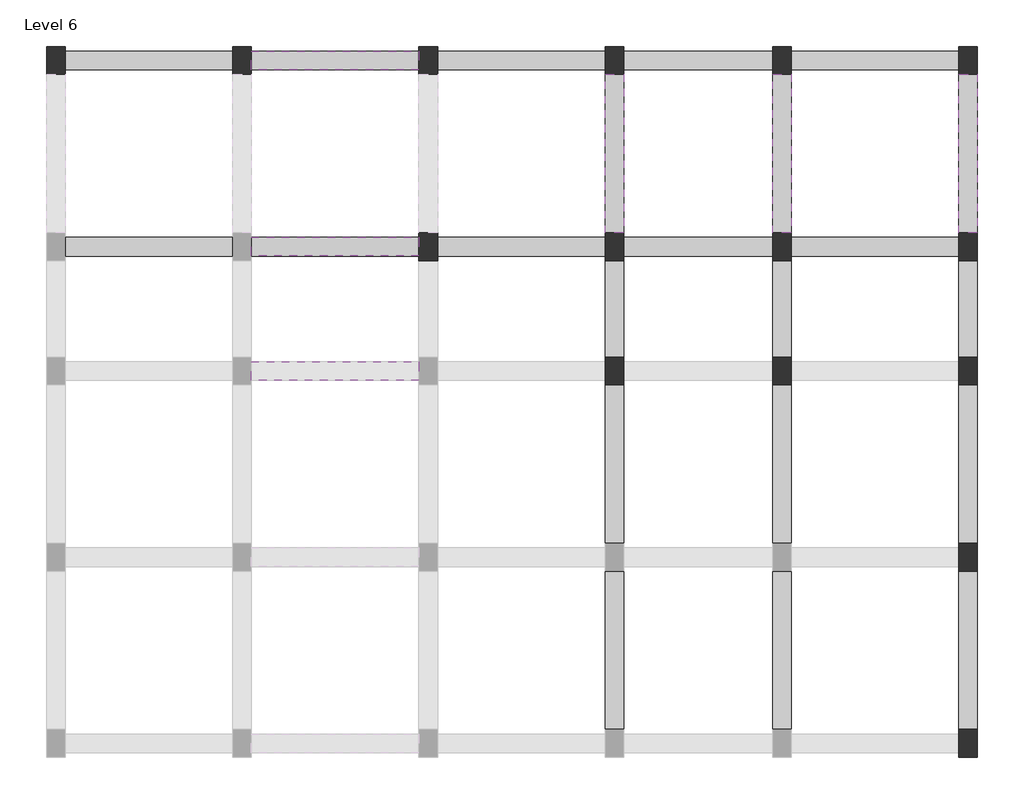
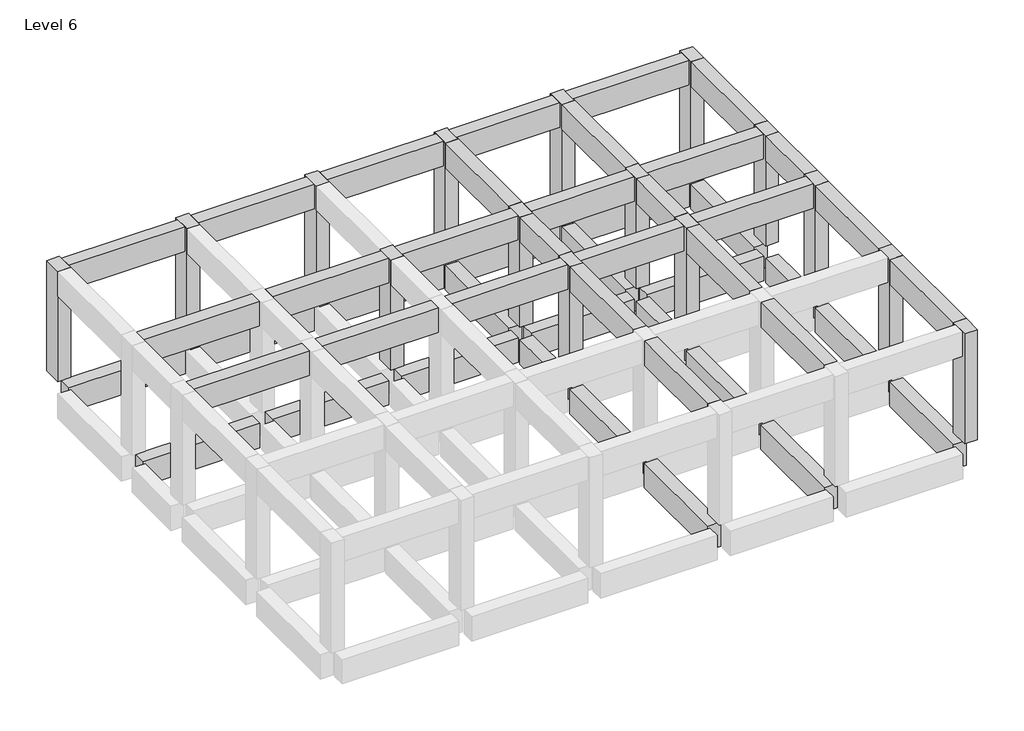
# One storey, part 2 of 2: 15 columns, 11 beams.
"""IFC4 building model written with IfcOpenShell, lengths in millimetres."""

from ifc_helpers import new_model, si_unit, frame, origin, place, context, project, spatial, polyline, outline, extrude, faceted_brep, element, save

model = new_model("IFC4")

# Units and contexts
model_context = context("Model", 3, world=origin())
ifc_project = project(units=[si_unit("LENGTHUNIT", "METRE", prefix="MILLI")], contexts=[model_context])

# Site, building, storey
site = spatial("IfcSite", under=ifc_project)
building = spatial("IfcBuilding", under=site)
storey = spatial("IfcBuildingStorey", under=building, Name="Level 6", Elevation=15240.0)

# Beams
placement = place(None, origin())
element("IfcBeam", 1, ObjectType="Concrete-Rectangular Beam : 12 x 24", at=placement, inside=storey, context=model_context, shape_type="SweptSolid", body=[
    extrude(outline(polyline([(2607.7603583, 15727.9119241), (2607.7603583, 15423.1119241), (-135.4396417, 15423.1119241), (-135.4396417, 15727.9119241), (2607.7603583, 15727.9119241)])), frame((0.0, 0.0, 14325.6), z_axis=(0.0, 0.0, 1.0), x_axis=(1.0, 0.0, 0.0)), (0.0, 0.0, 1.0), 609.6),
    extrude(outline(polyline([(-12022.6396417, 15423.1119241), (-12022.6396417, 15727.9119241), (-9279.4396417, 15727.9119241), (-9279.4396417, 15423.1119241), (-12022.6396417, 15423.1119241)])), frame((0.0, 0.0, 14325.6), z_axis=(0.0, 0.0, 1.0), x_axis=(1.0, 0.0, 0.0)), (0.0, 0.0, 1.0), 609.6),
    extrude(outline(polyline([(-8974.6396417, 15423.1119241), (-8974.6396417, 15727.9119241), (-6231.4396417, 15727.9119241), (-6231.4396417, 15423.1119241), (-8974.6396417, 15423.1119241)])), frame((0.0, 0.0, 14325.6), z_axis=(0.0, 0.0, 1.0), x_axis=(1.0, 0.0, 0.0)), (0.0, 0.0, 1.0), 609.6),
    extrude(outline(polyline([(-5926.6396417, 15423.1119241), (-5926.6396417, 15727.9119241), (-3183.4396417, 15727.9119241), (-3183.4396417, 15423.1119241), (-5926.6396417, 15423.1119241)])), frame((0.0, 0.0, 14325.6), z_axis=(0.0, 0.0, 1.0), x_axis=(1.0, 0.0, 0.0)), (0.0, 0.0, 1.0), 609.6),
    extrude(outline(polyline([(-2878.6396417, 15423.1119241), (-2878.6396417, 15727.9119241), (-440.2396417, 15727.9119241), (-440.2396417, 15423.1119241), (-2878.6396417, 15423.1119241)])), frame((0.0, 0.0, 14325.6), z_axis=(0.0, 0.0, 1.0), x_axis=(1.0, 0.0, 0.0)), (0.0, 0.0, 1.0), 609.6),
])
element("IfcBeam", 2, ObjectType="Concrete-Rectangular Beam : 12 x 24", at=placement, inside=storey, context=model_context, shape_type="SweptSolid", body=[
    extrude(outline(polyline([(2607.7603583, 18775.9119241), (2607.7603583, 18471.1119241), (-135.4396417, 18471.1119241), (-135.4396417, 18775.9119241), (2607.7603583, 18775.9119241)])), frame((0.0, 0.0, 14325.6), z_axis=(0.0, 0.0, 1.0), x_axis=(1.0, 0.0, 0.0)), (0.0, 0.0, 1.0), 609.6),
    extrude(outline(polyline([(-12022.6396417, 18471.1119241), (-12022.6396417, 18775.9119241), (-9279.4396417, 18775.9119241), (-9279.4396417, 18471.1119241), (-12022.6396417, 18471.1119241)])), frame((0.0, 0.0, 14325.6), z_axis=(0.0, 0.0, 1.0), x_axis=(1.0, 0.0, 0.0)), (0.0, 0.0, 1.0), 609.6),
    extrude(outline(polyline([(-8974.6396417, 18471.1119241), (-8974.6396417, 18775.9119241), (-6231.4396417, 18775.9119241), (-6231.4396417, 18471.1119241), (-8974.6396417, 18471.1119241)])), frame((0.0, 0.0, 14325.6), z_axis=(0.0, 0.0, 1.0), x_axis=(1.0, 0.0, 0.0)), (0.0, 0.0, 1.0), 609.6),
    extrude(outline(polyline([(-5926.6396417, 18471.1119241), (-5926.6396417, 18775.9119241), (-3183.4396417, 18775.9119241), (-3183.4396417, 18471.1119241), (-5926.6396417, 18471.1119241)])), frame((0.0, 0.0, 14325.6), z_axis=(0.0, 0.0, 1.0), x_axis=(1.0, 0.0, 0.0)), (0.0, 0.0, 1.0), 609.6),
    extrude(outline(polyline([(-2878.6396417, 18471.1119241), (-2878.6396417, 18775.9119241), (-440.2396417, 18775.9119241), (-440.2396417, 18471.1119241), (-2878.6396417, 18471.1119241)])), frame((0.0, 0.0, 14325.6), z_axis=(0.0, 0.0, 1.0), x_axis=(1.0, 0.0, 0.0)), (0.0, 0.0, 1.0), 609.6),
])
element("IfcBeam", 3, ObjectType="Concrete-Rectangular Beam : 12 x 24", at=placement, inside=storey, context=model_context, shape_type="SweptSolid", body=[
    extrude(outline(polyline([(-2878.6396417, 7672.8647757), (-3183.4396417, 7672.8647757), (-3183.4396417, 10263.6647757), (-2878.6396417, 10263.6647757), (-2878.6396417, 7672.8647757)])), frame((0.0, 0.0, 14325.6), z_axis=(0.0, 0.0, 1.0), x_axis=(1.0, 0.0, 0.0)), (0.0, 0.0, 1.0), 609.6),
    extrude(outline(polyline([(-3183.4396417, 18394.9119241), (-2878.6396417, 18394.9119241), (-2878.6396417, 15804.1119241), (-3183.4396417, 15804.1119241), (-3183.4396417, 18394.9119241)])), frame((0.0, 0.0, 14325.6), z_axis=(0.0, 0.0, 1.0), x_axis=(1.0, 0.0, 0.0)), (0.0, 0.0, 1.0), 609.6),
    extrude(outline(polyline([(-2878.6396417, 10720.8647757), (-3183.4396417, 10720.8647757), (-3183.4396417, 13311.6647757), (-2878.6396417, 13311.6647757), (-2878.6396417, 10720.8647757)])), frame((0.0, 0.0, 14325.6), z_axis=(0.0, 0.0, 1.0), x_axis=(1.0, 0.0, 0.0)), (0.0, 0.0, 1.0), 609.6),
    extrude(outline(polyline([(-2878.6396417, 13768.8647757), (-3183.4396417, 13768.8647757), (-3183.4396417, 15346.9119241), (-2878.6396417, 15346.9119241), (-2878.6396417, 13768.8647757)])), frame((0.0, 0.0, 14325.6), z_axis=(0.0, 0.0, 1.0), x_axis=(1.0, 0.0, 0.0)), (0.0, 0.0, 1.0), 609.6),
])
element("IfcBeam", 4, ObjectType="Concrete-Rectangular Beam : 12 x 24", at=placement, inside=storey, context=model_context, shape_type="SweptSolid", body=[
    extrude(outline(polyline([(-135.4396417, 7672.8647757), (-440.2396417, 7672.8647757), (-440.2396417, 10263.6647757), (-135.4396417, 10263.6647757), (-135.4396417, 7672.8647757)])), frame((0.0, 0.0, 14325.6), z_axis=(0.0, 0.0, 1.0), x_axis=(1.0, 0.0, 0.0)), (0.0, 0.0, 1.0), 609.6),
    extrude(outline(polyline([(-440.2396417, 18394.9119241), (-135.4396417, 18394.9119241), (-135.4396417, 15804.1119241), (-440.2396417, 15804.1119241), (-440.2396417, 18394.9119241)])), frame((0.0, 0.0, 14325.6), z_axis=(0.0, 0.0, 1.0), x_axis=(1.0, 0.0, 0.0)), (0.0, 0.0, 1.0), 609.6),
    extrude(outline(polyline([(-135.4396417, 10720.8647757), (-440.2396417, 10720.8647757), (-440.2396417, 13311.6647757), (-135.4396417, 13311.6647757), (-135.4396417, 10720.8647757)])), frame((0.0, 0.0, 14325.6), z_axis=(0.0, 0.0, 1.0), x_axis=(1.0, 0.0, 0.0)), (0.0, 0.0, 1.0), 609.6),
    extrude(outline(polyline([(-135.4396417, 13768.8647757), (-440.2396417, 13768.8647757), (-440.2396417, 15346.9119241), (-135.4396417, 15346.9119241), (-135.4396417, 13768.8647757)])), frame((0.0, 0.0, 14325.6), z_axis=(0.0, 0.0, 1.0), x_axis=(1.0, 0.0, 0.0)), (0.0, 0.0, 1.0), 609.6),
])
element("IfcBeam", 5, ObjectType="Concrete-Rectangular Beam : 12 x 24", at=placement, inside=storey, context=model_context, shape_type="SweptSolid", body=[
    extrude(outline(polyline([(2912.5603583, 7672.8647757), (2607.7603583, 7672.8647757), (2607.7603583, 10263.6647757), (2912.5603583, 10263.6647757), (2912.5603583, 7672.8647757)])), frame((0.0, 0.0, 14325.6), z_axis=(0.0, 0.0, 1.0), x_axis=(1.0, 0.0, 0.0)), (0.0, 0.0, 1.0), 609.6),
    extrude(outline(polyline([(2607.7603583, 18394.9119241), (2912.5603583, 18394.9119241), (2912.5603583, 15804.1119241), (2607.7603583, 15804.1119241), (2607.7603583, 18394.9119241)])), frame((0.0, 0.0, 14325.6), z_axis=(0.0, 0.0, 1.0), x_axis=(1.0, 0.0, 0.0)), (0.0, 0.0, 1.0), 609.6),
    extrude(outline(polyline([(2912.5603583, 10720.8647757), (2607.7603583, 10720.8647757), (2607.7603583, 13311.6647757), (2912.5603583, 13311.6647757), (2912.5603583, 10720.8647757)])), frame((0.0, 0.0, 14325.6), z_axis=(0.0, 0.0, 1.0), x_axis=(1.0, 0.0, 0.0)), (0.0, 0.0, 1.0), 609.6),
    extrude(outline(polyline([(2912.5603583, 13768.8647757), (2607.7603583, 13768.8647757), (2607.7603583, 15346.9119241), (2912.5603583, 15346.9119241), (2912.5603583, 13768.8647757)])), frame((0.0, 0.0, 14325.6), z_axis=(0.0, 0.0, 1.0), x_axis=(1.0, 0.0, 0.0)), (0.0, 0.0, 1.0), 609.6),
])
element("IfcBeam", 6, ObjectType="Concrete-Rectangular Beam : 12 x 24", at=placement, inside=storey, context=model_context, shape_type="SweptSolid", body=[
    extrude(outline(polyline([(2607.7603583, 13692.6647757), (2607.7603583, 13387.8647757), (-135.4396417, 13387.8647757), (-135.4396417, 13692.6647757), (2607.7603583, 13692.6647757)])), frame((0.0, 0.0, 17373.6), z_axis=(0.0, 0.0, 1.0), x_axis=(1.0, 0.0, 0.0)), (0.0, 0.0, 1.0), 609.6),
    extrude(outline(polyline([(-12022.6396417, 13387.8647757), (-12022.6396417, 13692.6647757), (-9279.4396417, 13692.6647757), (-9279.4396417, 13387.8647757), (-12022.6396417, 13387.8647757)])), frame((0.0, 0.0, 17373.6), z_axis=(0.0, 0.0, 1.0), x_axis=(1.0, 0.0, 0.0)), (0.0, 0.0, 1.0), 609.6),
    extrude(outline(polyline([(-8974.6396417, 13387.8647757), (-8974.6396417, 13692.6647757), (-6231.4396417, 13692.6647757), (-6231.4396417, 13387.8647757), (-8974.6396417, 13387.8647757)])), frame((0.0, 0.0, 17373.6), z_axis=(0.0, 0.0, 1.0), x_axis=(1.0, 0.0, 0.0)), (0.0, 0.0, 1.0), 609.6),
    extrude(outline(polyline([(-5926.6396417, 13387.8647757), (-5926.6396417, 13692.6647757), (-3183.4396417, 13692.6647757), (-3183.4396417, 13387.8647757), (-5926.6396417, 13387.8647757)])), frame((0.0, 0.0, 17373.6), z_axis=(0.0, 0.0, 1.0), x_axis=(1.0, 0.0, 0.0)), (0.0, 0.0, 1.0), 609.6),
    extrude(outline(polyline([(-2878.6396417, 13387.8647757), (-2878.6396417, 13692.6647757), (-440.2396417, 13692.6647757), (-440.2396417, 13387.8647757), (-2878.6396417, 13387.8647757)])), frame((0.0, 0.0, 17373.6), z_axis=(0.0, 0.0, 1.0), x_axis=(1.0, 0.0, 0.0)), (0.0, 0.0, 1.0), 609.6),
])
element("IfcBeam", 7, ObjectType="Concrete-Rectangular Beam : 12 x 24", at=placement, inside=storey, context=model_context, shape_type="SweptSolid", body=[
    extrude(outline(polyline([(2607.7603583, 15727.9119241), (2607.7603583, 15423.1119241), (-135.4396417, 15423.1119241), (-135.4396417, 15727.9119241), (2607.7603583, 15727.9119241)])), frame((0.0, 0.0, 17373.6), z_axis=(0.0, 0.0, 1.0), x_axis=(1.0, 0.0, 0.0)), (0.0, 0.0, 1.0), 609.6),
    extrude(outline(polyline([(-12022.6396417, 15423.1119241), (-12022.6396417, 15727.9119241), (-9279.4396417, 15727.9119241), (-9279.4396417, 15423.1119241), (-12022.6396417, 15423.1119241)])), frame((0.0, 0.0, 17373.6), z_axis=(0.0, 0.0, 1.0), x_axis=(1.0, 0.0, 0.0)), (0.0, 0.0, 1.0), 609.6),
    extrude(outline(polyline([(-8974.6396417, 15423.1119241), (-8974.6396417, 15727.9119241), (-6231.4396417, 15727.9119241), (-6231.4396417, 15423.1119241), (-8974.6396417, 15423.1119241)])), frame((0.0, 0.0, 17373.6), z_axis=(0.0, 0.0, 1.0), x_axis=(1.0, 0.0, 0.0)), (0.0, 0.0, 1.0), 609.6),
    extrude(outline(polyline([(-5926.6396417, 15423.1119241), (-5926.6396417, 15727.9119241), (-3183.4396417, 15727.9119241), (-3183.4396417, 15423.1119241), (-5926.6396417, 15423.1119241)])), frame((0.0, 0.0, 17373.6), z_axis=(0.0, 0.0, 1.0), x_axis=(1.0, 0.0, 0.0)), (0.0, 0.0, 1.0), 609.6),
    extrude(outline(polyline([(-2878.6396417, 15423.1119241), (-2878.6396417, 15727.9119241), (-440.2396417, 15727.9119241), (-440.2396417, 15423.1119241), (-2878.6396417, 15423.1119241)])), frame((0.0, 0.0, 17373.6), z_axis=(0.0, 0.0, 1.0), x_axis=(1.0, 0.0, 0.0)), (0.0, 0.0, 1.0), 609.6),
])
element("IfcBeam", 8, ObjectType="Concrete-Rectangular Beam : 12 x 24", at=placement, inside=storey, context=model_context, shape_type="SweptSolid", body=[
    extrude(outline(polyline([(2607.7603583, 18775.9119241), (2607.7603583, 18471.1119241), (-135.4396417, 18471.1119241), (-135.4396417, 18775.9119241), (2607.7603583, 18775.9119241)])), frame((0.0, 0.0, 17373.6), z_axis=(0.0, 0.0, 1.0), x_axis=(1.0, 0.0, 0.0)), (0.0, 0.0, 1.0), 609.6),
    extrude(outline(polyline([(-12022.6396417, 18471.1119241), (-12022.6396417, 18775.9119241), (-9279.4396417, 18775.9119241), (-9279.4396417, 18471.1119241), (-12022.6396417, 18471.1119241)])), frame((0.0, 0.0, 17373.6), z_axis=(0.0, 0.0, 1.0), x_axis=(1.0, 0.0, 0.0)), (0.0, 0.0, 1.0), 609.6),
    extrude(outline(polyline([(-8974.6396417, 18471.1119241), (-8974.6396417, 18775.9119241), (-6231.4396417, 18775.9119241), (-6231.4396417, 18471.1119241), (-8974.6396417, 18471.1119241)])), frame((0.0, 0.0, 17373.6), z_axis=(0.0, 0.0, 1.0), x_axis=(1.0, 0.0, 0.0)), (0.0, 0.0, 1.0), 609.6),
    extrude(outline(polyline([(-5926.6396417, 18471.1119241), (-5926.6396417, 18775.9119241), (-3183.4396417, 18775.9119241), (-3183.4396417, 18471.1119241), (-5926.6396417, 18471.1119241)])), frame((0.0, 0.0, 17373.6), z_axis=(0.0, 0.0, 1.0), x_axis=(1.0, 0.0, 0.0)), (0.0, 0.0, 1.0), 609.6),
    extrude(outline(polyline([(-2878.6396417, 18471.1119241), (-2878.6396417, 18775.9119241), (-440.2396417, 18775.9119241), (-440.2396417, 18471.1119241), (-2878.6396417, 18471.1119241)])), frame((0.0, 0.0, 17373.6), z_axis=(0.0, 0.0, 1.0), x_axis=(1.0, 0.0, 0.0)), (0.0, 0.0, 1.0), 609.6),
])
element("IfcBeam", 9, ObjectType="Concrete-Rectangular Beam : 12 x 24", at=placement, inside=storey, context=model_context, shape_type="SweptSolid", body=[
    extrude(outline(polyline([(-2878.6396417, 7672.8647757), (-3183.4396417, 7672.8647757), (-3183.4396417, 10263.6647757), (-2878.6396417, 10263.6647757), (-2878.6396417, 7672.8647757)])), frame((0.0, 0.0, 17373.6), z_axis=(0.0, 0.0, 1.0), x_axis=(1.0, 0.0, 0.0)), (0.0, 0.0, 1.0), 609.6),
    extrude(outline(polyline([(-3183.4396417, 18394.9119241), (-2878.6396417, 18394.9119241), (-2878.6396417, 15804.1119241), (-3183.4396417, 15804.1119241), (-3183.4396417, 18394.9119241)])), frame((0.0, 0.0, 17373.6), z_axis=(0.0, 0.0, 1.0), x_axis=(1.0, 0.0, 0.0)), (0.0, 0.0, 1.0), 609.6),
    extrude(outline(polyline([(-2878.6396417, 10720.8647757), (-3183.4396417, 10720.8647757), (-3183.4396417, 13311.6647757), (-2878.6396417, 13311.6647757), (-2878.6396417, 10720.8647757)])), frame((0.0, 0.0, 17373.6), z_axis=(0.0, 0.0, 1.0), x_axis=(1.0, 0.0, 0.0)), (0.0, 0.0, 1.0), 609.6),
    extrude(outline(polyline([(-2878.6396417, 13768.8647757), (-3183.4396417, 13768.8647757), (-3183.4396417, 15346.9119241), (-2878.6396417, 15346.9119241), (-2878.6396417, 13768.8647757)])), frame((0.0, 0.0, 17373.6), z_axis=(0.0, 0.0, 1.0), x_axis=(1.0, 0.0, 0.0)), (0.0, 0.0, 1.0), 609.6),
])
element("IfcBeam", 10, ObjectType="Concrete-Rectangular Beam : 12 x 24", at=placement, inside=storey, context=model_context, shape_type="SweptSolid", body=[
    extrude(outline(polyline([(-135.4396417, 7672.8647757), (-440.2396417, 7672.8647757), (-440.2396417, 10263.6647757), (-135.4396417, 10263.6647757), (-135.4396417, 7672.8647757)])), frame((0.0, 0.0, 17373.6), z_axis=(0.0, 0.0, 1.0), x_axis=(1.0, 0.0, 0.0)), (0.0, 0.0, 1.0), 609.6),
    extrude(outline(polyline([(-440.2396417, 18394.9119241), (-135.4396417, 18394.9119241), (-135.4396417, 15804.1119241), (-440.2396417, 15804.1119241), (-440.2396417, 18394.9119241)])), frame((0.0, 0.0, 17373.6), z_axis=(0.0, 0.0, 1.0), x_axis=(1.0, 0.0, 0.0)), (0.0, 0.0, 1.0), 609.6),
    extrude(outline(polyline([(-135.4396417, 10720.8647757), (-440.2396417, 10720.8647757), (-440.2396417, 13311.6647757), (-135.4396417, 13311.6647757), (-135.4396417, 10720.8647757)])), frame((0.0, 0.0, 17373.6), z_axis=(0.0, 0.0, 1.0), x_axis=(1.0, 0.0, 0.0)), (0.0, 0.0, 1.0), 609.6),
    extrude(outline(polyline([(-135.4396417, 13768.8647757), (-440.2396417, 13768.8647757), (-440.2396417, 15346.9119241), (-135.4396417, 15346.9119241), (-135.4396417, 13768.8647757)])), frame((0.0, 0.0, 17373.6), z_axis=(0.0, 0.0, 1.0), x_axis=(1.0, 0.0, 0.0)), (0.0, 0.0, 1.0), 609.6),
])
element("IfcBeam", 11, ObjectType="Concrete-Rectangular Beam : 12 x 24", at=placement, inside=storey, context=model_context, shape_type="SweptSolid", body=[
    extrude(outline(polyline([(2912.5603583, 7672.8647757), (2607.7603583, 7672.8647757), (2607.7603583, 10263.6647757), (2912.5603583, 10263.6647757), (2912.5603583, 7672.8647757)])), frame((0.0, 0.0, 17373.6), z_axis=(0.0, 0.0, 1.0), x_axis=(1.0, 0.0, 0.0)), (0.0, 0.0, 1.0), 609.6),
    extrude(outline(polyline([(2607.7603583, 18394.9119241), (2912.5603583, 18394.9119241), (2912.5603583, 15804.1119241), (2607.7603583, 15804.1119241), (2607.7603583, 18394.9119241)])), frame((0.0, 0.0, 17373.6), z_axis=(0.0, 0.0, 1.0), x_axis=(1.0, 0.0, 0.0)), (0.0, 0.0, 1.0), 609.6),
    extrude(outline(polyline([(2912.5603583, 10720.8647757), (2607.7603583, 10720.8647757), (2607.7603583, 13311.6647757), (2912.5603583, 13311.6647757), (2912.5603583, 10720.8647757)])), frame((0.0, 0.0, 17373.6), z_axis=(0.0, 0.0, 1.0), x_axis=(1.0, 0.0, 0.0)), (0.0, 0.0, 1.0), 609.6),
    extrude(outline(polyline([(2912.5603583, 13768.8647757), (2607.7603583, 13768.8647757), (2607.7603583, 15346.9119241), (2912.5603583, 15346.9119241), (2912.5603583, 13768.8647757)])), frame((0.0, 0.0, 17373.6), z_axis=(0.0, 0.0, 1.0), x_axis=(1.0, 0.0, 0.0)), (0.0, 0.0, 1.0), 609.6),
])

# Columns
element("IfcColumn", 12, ObjectType="Concrete-Rectangular-Column : c1", at=placement, inside=storey, context=model_context, shape_type="SweptSolid", body=[
    extrude(outline(polyline([(2607.7603583, 7215.6647757), (2607.7603583, 7672.8647757), (2912.5603583, 7672.8647757), (2912.5603583, 7215.6647757), (2607.7603583, 7215.6647757)])), frame((0.0, 0.0, 15240.0), z_axis=(0.0, 0.0, 1.0), x_axis=(1.0, 0.0, 0.0)), (0.0, 0.0, 1.0), 2743.2),
])
element("IfcColumn", 13, ObjectType="Concrete-Rectangular-Column : c1", at=placement, inside=storey, context=model_context, shape_type="Brep", body=[
    faceted_brep([(2607.7603583, 10263.6647757, 15240.0), (2607.7603583, 10720.8647757, 15240.0), (2912.5603583, 10720.8647757, 15240.0), (2912.5603583, 10263.6647757, 15240.0), (2607.7603583, 10263.6647757, 17983.2), (2607.7603583, 10720.8647757, 17983.2), (2607.7603583, 10720.8647757, 17373.6), (2607.7603583, 10263.6647757, 17373.6), (2912.5603583, 10720.8647757, 17983.2), (2912.5603583, 10720.8647757, 17373.6), (2912.5603583, 10263.6647757, 17983.2), (2912.5603583, 10263.6647757, 17373.6)], [[[0, 1, 2, 3]], [[4, 5, 6, 1, 0, 7]], [[5, 8, 9, 2, 1, 6]], [[8, 10, 11, 3, 2, 9]], [[10, 4, 7, 0, 3, 11]], [[4, 10, 8, 5]]]),
])
element("IfcColumn", 14, ObjectType="Concrete-Rectangular-Column : c1", at=placement, inside=storey, context=model_context, shape_type="Brep", body=[
    faceted_brep([(-3183.4396417, 13311.6647757, 15240.0), (-3183.4396417, 13768.8647757, 15240.0), (-2878.6396417, 13768.8647757, 15240.0), (-2878.6396417, 13311.6647757, 15240.0), (-3183.4396417, 13311.6647757, 17983.2), (-3183.4396417, 13387.8647757, 17983.2), (-3183.4396417, 13692.6647757, 17983.2), (-3183.4396417, 13768.8647757, 17983.2), (-3183.4396417, 13768.8647757, 17373.6), (-3183.4396417, 13311.6647757, 17373.6), (-2878.6396417, 13768.8647757, 17983.2), (-2878.6396417, 13768.8647757, 17373.6), (-2878.6396417, 13692.6647757, 17983.2), (-2878.6396417, 13387.8647757, 17983.2), (-2878.6396417, 13311.6647757, 17983.2), (-2878.6396417, 13311.6647757, 17373.6)], [[[0, 1, 2, 3]], [[4, 5, 6, 7, 8, 1, 0, 9]], [[7, 10, 11, 2, 1, 8]], [[10, 12, 13, 14, 15, 3, 2, 11]], [[14, 4, 9, 0, 3, 15]], [[4, 14, 13, 12, 10, 7, 6, 5]]]),
])
element("IfcColumn", 15, ObjectType="Concrete-Rectangular-Column : c1", at=placement, inside=storey, context=model_context, shape_type="Brep", body=[
    faceted_brep([(-440.2396417, 13311.6647757, 15240.0), (-440.2396417, 13768.8647757, 15240.0), (-135.4396417, 13768.8647757, 15240.0), (-135.4396417, 13311.6647757, 15240.0), (-440.2396417, 13311.6647757, 17983.2), (-440.2396417, 13387.8647757, 17983.2), (-440.2396417, 13692.6647757, 17983.2), (-440.2396417, 13768.8647757, 17983.2), (-440.2396417, 13768.8647757, 17373.6), (-440.2396417, 13311.6647757, 17373.6), (-135.4396417, 13768.8647757, 17983.2), (-135.4396417, 13768.8647757, 17373.6), (-135.4396417, 13692.6647757, 17983.2), (-135.4396417, 13387.8647757, 17983.2), (-135.4396417, 13311.6647757, 17983.2), (-135.4396417, 13311.6647757, 17373.6)], [[[0, 1, 2, 3]], [[4, 5, 6, 7, 8, 1, 0, 9]], [[7, 10, 11, 2, 1, 8]], [[10, 12, 13, 14, 15, 3, 2, 11]], [[14, 4, 9, 0, 3, 15]], [[4, 14, 13, 12, 10, 7, 6, 5]]]),
])
element("IfcColumn", 16, ObjectType="Concrete-Rectangular-Column : c1", at=placement, inside=storey, context=model_context, shape_type="Brep", body=[
    faceted_brep([(2607.7603583, 13311.6647757, 15240.0), (2607.7603583, 13768.8647757, 15240.0), (2912.5603583, 13768.8647757, 15240.0), (2912.5603583, 13311.6647757, 15240.0), (2607.7603583, 13311.6647757, 17983.2), (2607.7603583, 13768.8647757, 17983.2), (2607.7603583, 13768.8647757, 17373.6), (2607.7603583, 13311.6647757, 17373.6), (2912.5603583, 13768.8647757, 17983.2), (2912.5603583, 13768.8647757, 17373.6), (2912.5603583, 13311.6647757, 17983.2), (2912.5603583, 13311.6647757, 17373.6)], [[[0, 1, 2, 3]], [[4, 5, 6, 1, 0, 7]], [[5, 8, 9, 2, 1, 6]], [[8, 10, 11, 3, 2, 9]], [[10, 4, 7, 0, 3, 11]], [[4, 10, 8, 5]]]),
])
element("IfcColumn", 17, ObjectType="Concrete-Rectangular-Column : c1", at=placement, inside=storey, context=model_context, shape_type="Brep", body=[
    faceted_brep([(-6231.4396417, 15346.9119241, 15240.0), (-6231.4396417, 15804.1119241, 15240.0), (-5926.6396417, 15804.1119241, 15240.0), (-5926.6396417, 15346.9119241, 15240.0), (-6231.4396417, 15346.9119241, 17983.2), (-6231.4396417, 15423.1119241, 17983.2), (-6231.4396417, 15727.9119241, 17983.2), (-6231.4396417, 15804.1119241, 17983.2), (-6231.4396417, 15804.1119241, 17373.6), (-6231.4396417, 15346.9119241, 17373.6), (-5926.6396417, 15804.1119241, 17983.2), (-5926.6396417, 15804.1119241, 17373.6), (-5926.6396417, 15727.9119241, 17983.2), (-5926.6396417, 15423.1119241, 17983.2), (-5926.6396417, 15346.9119241, 17983.2), (-5926.6396417, 15346.9119241, 17373.6)], [[[0, 1, 2, 3]], [[4, 5, 6, 7, 8, 1, 0, 9]], [[7, 10, 11, 2, 1, 8]], [[10, 12, 13, 14, 15, 3, 2, 11]], [[14, 4, 9, 0, 3, 15]], [[4, 14, 13, 12, 10, 7, 6, 5]]]),
])
element("IfcColumn", 18, ObjectType="Concrete-Rectangular-Column : c1", at=placement, inside=storey, context=model_context, shape_type="Brep", body=[
    faceted_brep([(-3183.4396417, 15346.9119241, 15240.0), (-3183.4396417, 15804.1119241, 15240.0), (-2878.6396417, 15804.1119241, 15240.0), (-2878.6396417, 15346.9119241, 15240.0), (-3183.4396417, 15346.9119241, 17983.2), (-3183.4396417, 15423.1119241, 17983.2), (-3183.4396417, 15727.9119241, 17983.2), (-3183.4396417, 15804.1119241, 17983.2), (-3183.4396417, 15804.1119241, 17373.6), (-3183.4396417, 15346.9119241, 17373.6), (-2878.6396417, 15804.1119241, 17983.2), (-2878.6396417, 15804.1119241, 17373.6), (-2878.6396417, 15727.9119241, 17983.2), (-2878.6396417, 15423.1119241, 17983.2), (-2878.6396417, 15346.9119241, 17983.2), (-2878.6396417, 15346.9119241, 17373.6)], [[[0, 1, 2, 3]], [[4, 5, 6, 7, 8, 1, 0, 9]], [[7, 10, 11, 2, 1, 8]], [[10, 12, 13, 14, 15, 3, 2, 11]], [[14, 4, 9, 0, 3, 15]], [[4, 14, 13, 12, 10, 7, 6, 5]]]),
])
element("IfcColumn", 19, ObjectType="Concrete-Rectangular-Column : c1", at=placement, inside=storey, context=model_context, shape_type="Brep", body=[
    faceted_brep([(-440.2396417, 15346.9119241, 15240.0), (-440.2396417, 15804.1119241, 15240.0), (-135.4396417, 15804.1119241, 15240.0), (-135.4396417, 15346.9119241, 15240.0), (-440.2396417, 15346.9119241, 17983.2), (-440.2396417, 15423.1119241, 17983.2), (-440.2396417, 15727.9119241, 17983.2), (-440.2396417, 15804.1119241, 17983.2), (-440.2396417, 15804.1119241, 17373.6), (-440.2396417, 15346.9119241, 17373.6), (-135.4396417, 15804.1119241, 17983.2), (-135.4396417, 15804.1119241, 17373.6), (-135.4396417, 15727.9119241, 17983.2), (-135.4396417, 15423.1119241, 17983.2), (-135.4396417, 15346.9119241, 17983.2), (-135.4396417, 15346.9119241, 17373.6)], [[[0, 1, 2, 3]], [[4, 5, 6, 7, 8, 1, 0, 9]], [[7, 10, 11, 2, 1, 8]], [[10, 12, 13, 14, 15, 3, 2, 11]], [[14, 4, 9, 0, 3, 15]], [[4, 14, 13, 12, 10, 7, 6, 5]]]),
])
element("IfcColumn", 20, ObjectType="Concrete-Rectangular-Column : c1", at=placement, inside=storey, context=model_context, shape_type="Brep", body=[
    faceted_brep([(2607.7603583, 15346.9119241, 15240.0), (2607.7603583, 15804.1119241, 15240.0), (2912.5603583, 15804.1119241, 15240.0), (2912.5603583, 15346.9119241, 15240.0), (2607.7603583, 15346.9119241, 17983.2), (2607.7603583, 15804.1119241, 17983.2), (2607.7603583, 15804.1119241, 17373.6), (2607.7603583, 15346.9119241, 17373.6), (2912.5603583, 15804.1119241, 17983.2), (2912.5603583, 15804.1119241, 17373.6), (2912.5603583, 15346.9119241, 17983.2), (2912.5603583, 15346.9119241, 17373.6)], [[[0, 1, 2, 3]], [[4, 5, 6, 1, 0, 7]], [[5, 8, 9, 2, 1, 6]], [[8, 10, 11, 3, 2, 9]], [[10, 4, 7, 0, 3, 11]], [[4, 10, 8, 5]]]),
])
element("IfcColumn", 21, ObjectType="Concrete-Rectangular-Column : c1", at=placement, inside=storey, context=model_context, shape_type="SweptSolid", body=[
    extrude(outline(polyline([(-12327.4396417, 18394.9119241), (-12327.4396417, 18852.1119241), (-12022.6396417, 18852.1119241), (-12022.6396417, 18394.9119241), (-12327.4396417, 18394.9119241)])), frame((0.0, 0.0, 15240.0), z_axis=(0.0, 0.0, 1.0), x_axis=(1.0, 0.0, 0.0)), (0.0, 0.0, 1.0), 2743.2),
])
element("IfcColumn", 22, ObjectType="Concrete-Rectangular-Column : c1", at=placement, inside=storey, context=model_context, shape_type="Brep", body=[
    faceted_brep([(-9279.4396417, 18394.9119241, 15240.0), (-9279.4396417, 18852.1119241, 15240.0), (-8974.6396417, 18852.1119241, 15240.0), (-8974.6396417, 18394.9119241, 15240.0), (-9279.4396417, 18394.9119241, 17983.2), (-9279.4396417, 18471.1119241, 17983.2), (-9279.4396417, 18775.9119241, 17983.2), (-9279.4396417, 18852.1119241, 17983.2), (-8974.6396417, 18852.1119241, 17983.2), (-8974.6396417, 18775.9119241, 17983.2), (-8974.6396417, 18471.1119241, 17983.2), (-8974.6396417, 18394.9119241, 17983.2)], [[[0, 1, 2, 3]], [[4, 5, 6, 7, 1, 0]], [[7, 8, 2, 1]], [[8, 9, 10, 11, 3, 2]], [[11, 4, 0, 3]], [[4, 11, 10, 9, 8, 7, 6, 5]]]),
])
element("IfcColumn", 23, ObjectType="Concrete-Rectangular-Column : c1", at=placement, inside=storey, context=model_context, shape_type="Brep", body=[
    faceted_brep([(-6231.4396417, 18394.9119241, 15240.0), (-6231.4396417, 18852.1119241, 15240.0), (-5926.6396417, 18852.1119241, 15240.0), (-5926.6396417, 18394.9119241, 15240.0), (-6231.4396417, 18394.9119241, 17983.2), (-6231.4396417, 18471.1119241, 17983.2), (-6231.4396417, 18775.9119241, 17983.2), (-6231.4396417, 18852.1119241, 17983.2), (-5926.6396417, 18852.1119241, 17983.2), (-5926.6396417, 18775.9119241, 17983.2), (-5926.6396417, 18471.1119241, 17983.2), (-5926.6396417, 18394.9119241, 17983.2)], [[[0, 1, 2, 3]], [[4, 5, 6, 7, 1, 0]], [[7, 8, 2, 1]], [[8, 9, 10, 11, 3, 2]], [[11, 4, 0, 3]], [[4, 11, 10, 9, 8, 7, 6, 5]]]),
])
element("IfcColumn", 24, ObjectType="Concrete-Rectangular-Column : c1", at=placement, inside=storey, context=model_context, shape_type="Brep", body=[
    faceted_brep([(-3183.4396417, 18394.9119241, 15240.0), (-3183.4396417, 18852.1119241, 15240.0), (-2878.6396417, 18852.1119241, 15240.0), (-2878.6396417, 18394.9119241, 15240.0), (-3183.4396417, 18394.9119241, 17983.2), (-3183.4396417, 18471.1119241, 17983.2), (-3183.4396417, 18775.9119241, 17983.2), (-3183.4396417, 18852.1119241, 17983.2), (-2878.6396417, 18852.1119241, 17983.2), (-2878.6396417, 18775.9119241, 17983.2), (-2878.6396417, 18471.1119241, 17983.2), (-2878.6396417, 18394.9119241, 17983.2)], [[[0, 1, 2, 3]], [[4, 5, 6, 7, 1, 0]], [[7, 8, 2, 1]], [[8, 9, 10, 11, 3, 2]], [[11, 4, 0, 3]], [[4, 11, 10, 9, 8, 7, 6, 5]]]),
])
element("IfcColumn", 25, ObjectType="Concrete-Rectangular-Column : c1", at=placement, inside=storey, context=model_context, shape_type="Brep", body=[
    faceted_brep([(-440.2396417, 18394.9119241, 15240.0), (-440.2396417, 18852.1119241, 15240.0), (-135.4396417, 18852.1119241, 15240.0), (-135.4396417, 18394.9119241, 15240.0), (-440.2396417, 18394.9119241, 17983.2), (-440.2396417, 18471.1119241, 17983.2), (-440.2396417, 18775.9119241, 17983.2), (-440.2396417, 18852.1119241, 17983.2), (-135.4396417, 18852.1119241, 17983.2), (-135.4396417, 18775.9119241, 17983.2), (-135.4396417, 18471.1119241, 17983.2), (-135.4396417, 18394.9119241, 17983.2)], [[[0, 1, 2, 3]], [[4, 5, 6, 7, 1, 0]], [[7, 8, 2, 1]], [[8, 9, 10, 11, 3, 2]], [[11, 4, 0, 3]], [[4, 11, 10, 9, 8, 7, 6, 5]]]),
])
element("IfcColumn", 26, ObjectType="Concrete-Rectangular-Column : c1", at=placement, inside=storey, context=model_context, shape_type="SweptSolid", body=[
    extrude(outline(polyline([(2607.7603583, 18394.9119241), (2607.7603583, 18852.1119241), (2912.5603583, 18852.1119241), (2912.5603583, 18394.9119241), (2607.7603583, 18394.9119241)])), frame((0.0, 0.0, 15240.0), z_axis=(0.0, 0.0, 1.0), x_axis=(1.0, 0.0, 0.0)), (0.0, 0.0, 1.0), 2743.2),
])

save(model, "model.ifc")

# Revit data of these elements
# Type "Concrete-Rectangular Beam : 12 x 24"
#   Assembly Code = "B10"
#   Length [instance default] = 5' - 0"
#   b = 1' - 0"
#   h = 2' - 0"
#   Structural Material [instance default] = Concrete, Cast-in-Place gray
# Type "Concrete-Rectangular-Column : c1"
#   Assembly Code = "B10"
#   b = 1' - 0"
#   h = 1' - 6"
#   Structural Material [instance default] = Concrete, Cast-in-Place gray
# Elements 1, 2, 3, 4, 5, 6, 7, 8, 9, 10, 11 (IfcBeam, "Concrete-Rectangular Beam : 12 x 24")
#   Structural Material = Concrete, Cast-in-Place gray
#   Phase Created = New Construction
#   Materials on its faces: "Concrete, Cast-in-Place gray"
# Elements 12, 13, 14, 15, 16, 17, 18, 19, 20, 21, 22, 23, 24, 25, 26 (IfcColumn, "Concrete-Rectangular-Column : c1")
#   Comments = ""
#   Structural Material = Concrete, Cast-in-Place gray
#   Phase Created = New Construction
#   Materials on its faces: "Concrete, Cast-in-Place gray"
# Materials
#   "Concrete, Cast-in-Place gray": class "Concrete", colour RGB 192 192 192, transparency 0, Description = "Cast-in-place concrete", Cost = 0
